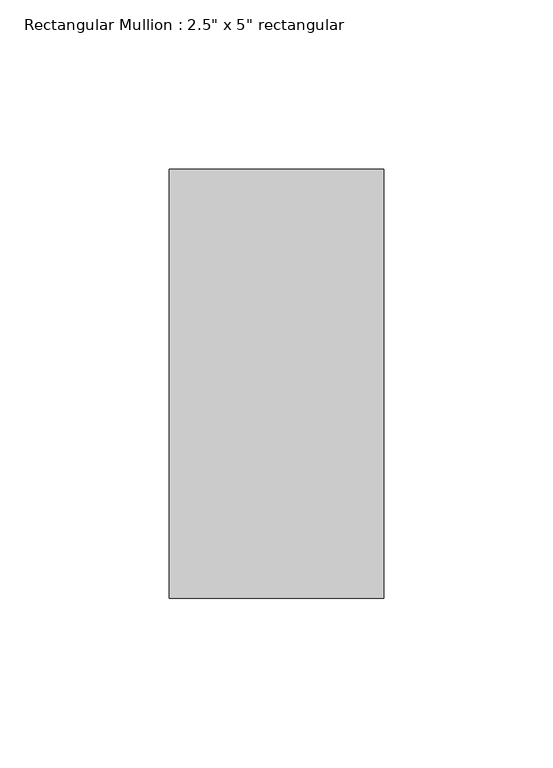
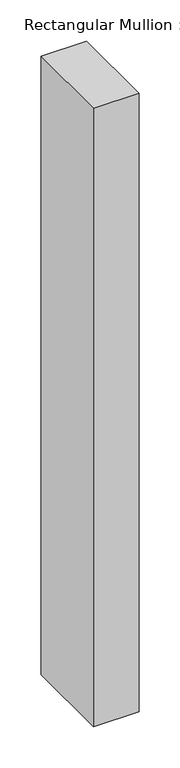
"""IFC4 building model written with IfcOpenShell, lengths in millimetres: member geometry."""

from ifc_helpers import new_model, si_unit, frame, origin, place, context, project, spatial, polyline, outline, extrude, source, transform, mapped, element, save


def member_238a442c(model_context):
    return source(origin(), model_context, "Body", "SweptSolid", [
        extrude(outline(polyline([(0.0, 63.5), (0.0, -63.5), (-63.5, -63.5), (-63.5, 63.5), (0.0, 63.5)])), frame((0.0, 0.0, -914.0980012), z_axis=(0.0, 0.0, 1.0), x_axis=(1.0, 0.0, 0.0)), (0.0, 0.0, 1.0), 914.0980012),
    ])


if __name__ == "__main__":
    model = new_model("IFC4")
    model_context = context("Model", 3, world=origin())
    ifc_project = project(units=[si_unit("LENGTHUNIT", "METRE", prefix="MILLI")], contexts=[model_context])
    site = spatial("IfcSite", under=ifc_project)
    building = spatial("IfcBuilding", under=site)
    placement = place(None, origin())
    member_shape = member_238a442c(model_context)
    element("IfcMember", 1, ObjectType="Rectangular Mullion : 2.5\" x 5\" rectangular", at=placement, inside=building, context=model_context, shape_type="MappedRepresentation", body=[
        mapped(member_shape, transform((0.0, 0.0, 0.0), x_axis=(1.0, 0.0, 0.0), y_axis=(0.0, 1.0, 0.0), z_axis=(0.0, 0.0, 1.0))),
    ])
    save(model, "model.ifc")

# Revit data of these elements
# Type "Rectangular Mullion : 2.5\" x 5\" rectangular"
#   built-in parameter 1007304 = 0.416667 (stored number, unit not read)
#   built-in parameter 1007301 = 0.104167 (stored number, unit not read)
#   built-in parameter 1007300 = 0.104167 (stored number, unit not read)
# Element 1 (IfcMember, "Rectangular Mullion : 2.5\" x 5\" rectangular")
#   Materials on its faces: "Aluminum"
# Materials
#   "Aluminum": class "Metal", colour RGB 247 247 247, transparency 0, Description = "Aluminum 6061", Cost = 0
